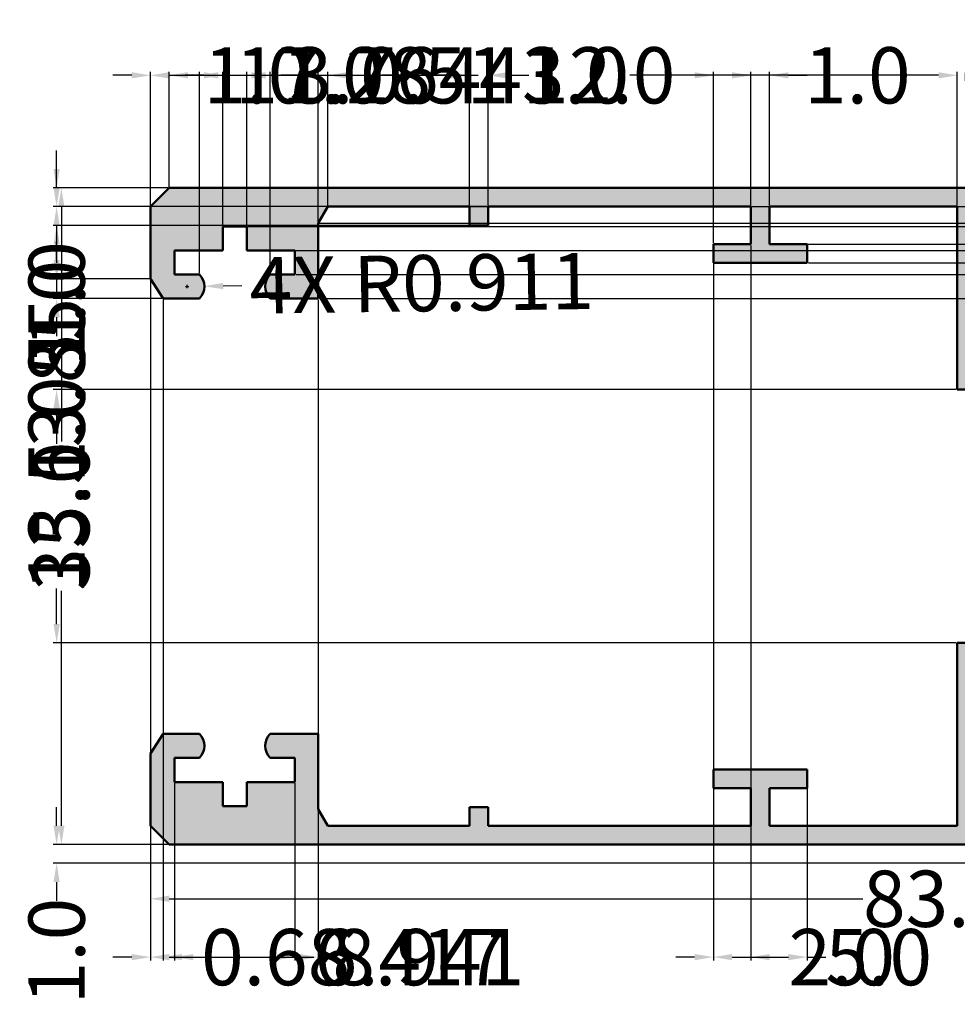
# Model space of a CAD drawing. Units: millimetres. Extents: x 9 to 262, y -226 to 104.
# Tile 3 of 4: x 119 to 169, y 13 to 66. Entities that reach past the tile are written whole.
import ezdxf

# ---------------------------------------------------------------- set-up
doc = ezdxf.new("R2010")
doc.units = ezdxf.units.MM
doc.header["$MEASUREMENT"] = 0
for name, color, linetype, lineweight in [('M-DIMS', 2, 'Continuous', 25), ('M-HATC', 9, 'Continuous', 18), ('M-OUTL', 7, 'Continuous', 50)]:
    doc.layers.add(name, color=color, linetype=linetype, lineweight=lineweight)
doc.styles.get("Standard").update_dxf_attribs({"font": 'arial.ttf'})
doc.dimstyles.get("Standard").update_dxf_attribs({"dimtxt": 3, "dimasz": 1, "dimexe": 0.18, "dimexo": 0.0625, "dimgap": 0.09, "dimtad": 0, "dimdec": 1, "dimzin": 0, "dimdsep": 46, "dimtxsty": 'Standard', "dimcen": 0.09, "dimadec": 0, "dimazin": 0, "dimtfac": 1, "dimtdec": 1, "dimtofl": 0, "dimtmove": 0, "dimatfit": 3, "dimfxl": 1, "dimtolj": 1, "dimtzin": 0, "dimarcsym": 0})

# ---------------------------------------------------------------- blocks, each defined once
blk = doc.blocks.new('*D3')
at = {"layer": 'Defpoints', "color": 0, "transparency": 16777216}
for p in [(126.103, 21.114), (210.003, 21.345), (126.103, 18.955)]:
    blk.add_point(p, dxfattribs=at)
at = {"layer": 'M-DIMS', "color": 0, "lineweight": -2, "transparency": 16777216}
for p, q in [((126.103, 21.051), (126.103, 18.775)), ((210.003, 21.282), (210.003, 18.775)), ((127.103, 18.955), (164.062, 18.955)), ((209.003, 18.955), (172.045, 18.955))]:
    blk.add_line(p, q, dxfattribs=at)
at = {"layer": 'M-DIMS', "color": 0, "transparency": 16777216}
for points in [[(127.103, 19.122), (127.103, 18.788), (126.103, 18.955)], [(209.003, 19.122), (209.003, 18.788), (210.003, 18.955)]]:
    blk.add_solid(points, dxfattribs=at)
at = {"layer": 'M-DIMS', "color": 0, "transparency": 16777216, "insert": (168.053, 18.955), "char_height": 3, "attachment_point": 5}
blk.add_mtext('\\A1;83.9', dxfattribs=at)
blk = doc.blocks.new('*D4')
at = {"layer": 'Defpoints', "color": 0, "transparency": 16777216}
for p in [(127.103, 56.845), (121.354, 21.845), (127.103, 21.845)]:
    blk.add_point(p, dxfattribs=at)
at = {"layer": 'M-DIMS', "color": 0, "lineweight": -2, "transparency": 16777216}
for p, q in [((127.041, 56.845), (121.174, 56.845)), ((121.354, 55.845), (121.354, 43.325)), ((121.354, 22.845), (121.354, 35.365)), ((127.041, 21.845), (121.174, 21.845))]:
    blk.add_line(p, q, dxfattribs=at)
at = {"layer": 'M-DIMS', "color": 0, "transparency": 16777216}
for points in [[(121.188, 55.845), (121.521, 55.845), (121.354, 56.845)], [(121.188, 22.845), (121.521, 22.845), (121.354, 21.845)]]:
    blk.add_solid(points, dxfattribs=at)
at = {"layer": 'M-DIMS', "color": 0, "transparency": 16777216, "insert": (121.354, 39.345), "char_height": 3, "attachment_point": 5, "rotation": 90}
blk.add_mtext('\\A1;35.0', dxfattribs=at)
blk = doc.blocks.new('PROFILE-SASH')
for p, q in [((66.477, 36), (68.209, 37)), ((68.209, 37), (83.4, 37)), ((1, 36), (0, 35)), ((1, 36), (66.477, 36)), ((68, 35.724), (68.477, 36)), ((68, 35.724), (68, 1.275)), ((68.477, 36), (75.189, 36)), ((75.189, 36), (75.189, 33.5)), ((76.189, 36), (76.189, 33.5)), ((76.189, 36), (81.9, 36)), ((81.9, 36), (81.9, 32)), ((82.9, 36), (82.9, 32)), ((82.9, 36), (83.4, 36)), ((0, 35), (0, 31.15)), ((8.941, 34.12), (9.449, 35)), ((9.449, 35), (17, 35)), ((17, 35), (17, 34)), ((18, 35), (18, 34)), ((18, 35), (32, 35)), ((32, 35), (32, 33)), ((33, 35), (33, 33)), ((33, 35), (33, 33)), ((33, 35), (43, 35)), ((43, 35), (43, 25.25)), ((44, 35), (44, 28.25)), ((44, 35), (54, 35)), ((54, 35), (54, 34.5)), ((55, 35), (55, 34.5)), ((55, 35), (67, 35)), ((55, 35), (66.477, 35)), ((67, 35), (67, 2)), ((8.941, 30.101), (8.941, 34.12)), ((3.851, 32.668), (3.851, 33.951)), ((3.851, 33.951), (5.134, 33.951)), ((5.134, 32.668), (5.134, 33.951)), ((17, 34), (18, 34)), ((1.284, 31.384), (1.284, 32.668)), ((1.284, 31.384), (1.284, 32.668)), ((1.284, 32.668), (3.851, 32.668)), ((7.701, 32.668), (5.134, 32.668)), ((7.701, 31.384), (7.701, 32.668)), ((30, 32), (30, 33)), ((30, 33), (32, 33)), ((33, 33), (35, 33)), ((35, 33), (35, 32)), ((32, 32), (30, 32)), ((35, 32), (32, 32)), ((0, 31.15), (0.685, 30.101)), ((2.61, 31.384), (1.284, 31.384)), ((6.374, 31.384), (7.701, 31.384)), ((0.685, 30.101), (2.61, 30.101)), ((6.374, 30.101), (8.941, 30.101)), ((44, 28.25), (49, 28.25)), ((49, 28.25), (49, 8.75)), ((44, 27.25), (48, 27.25)), ((44, 27.25), (44, 25.25)), ((48, 27.25), (48, 9.75)), ((43, 25.25), (44, 25.25)), ((43, 11.75), (44, 11.75)), ((43, 11.75), (43, 2)), ((44, 11.75), (44, 9.75)), ((48, 9.75), (44, 9.75)), ((49, 8.75), (44, 8.75)), ((44, 8.75), (44, 2)), ((0, 5.85), (0.685, 6.899)), ((0.685, 6.899), (2.61, 6.899)), ((6.374, 6.899), (8.941, 6.899)), ((8.941, 6.899), (8.941, 2.879)), ((0, 5.85), (0, 2)), ((1.284, 5.615), (1.284, 4.332)), ((2.61, 5.615), (1.284, 5.615)), ((1.284, 5.615), (1.284, 4.332)), ((6.374, 5.615), (7.701, 5.615)), ((7.701, 5.615), (7.701, 4.332)), ((32, 5), (30, 5)), ((30, 5), (30, 4)), ((35, 5), (32, 5)), ((35, 4), (35, 5)), ((81.9, 5), (81.9, 1)), ((82.9, 5), (82.9, 1)), ((1.284, 4.332), (3.851, 4.332)), ((3.851, 4.332), (3.851, 3.049)), ((7.701, 4.332), (5.134, 4.332)), ((5.134, 4.332), (5.134, 3.049)), ((30, 4), (32, 4)), ((32, 4), (32, 2)), ((33, 2), (33, 4)), ((33, 4), (35, 4)), ((33, 4), (33, 2)), ((75.189, 3.5), (75.189, 1)), ((76.189, 3.5), (76.189, 1)), ((3.851, 3.049), (5.134, 3.049)), ((8.941, 2.879), (9.449, 2)), ((17, 3), (18, 3)), ((17, 3), (17, 2)), ((18, 3), (18, 2)), ((54, 2.5), (54, 2)), ((55, 2.5), (55, 2)), ((0, 2), (1, 1)), ((9.449, 2), (17, 2)), ((18, 2), (32, 2)), ((33, 2), (43, 2)), ((44, 2), (54, 2)), ((44, 2), (54, 2)), ((55, 2), (67, 2)), ((55, 2), (66.477, 2)), ((68, 1.275), (68.477, 1)), ((1, 1), (66.477, 1)), ((66.477, 1), (68.209, 0)), ((68.477, 1), (75.189, 1)), ((76.189, 1), (81.9, 1)), ((76.189, 1), (81.9, 1)), ((82.9, 1), (83.4, 1)), ((82.9, 1), (83.4, 1)), ((68.209, 0), (83.4, 0))]:
    blk.add_line(p, q)
for centre, radius, start, end in [((83.4, 36.5), 0.5, 270, 90), ((54.5, 34.5), 0.5, 180, 0), ((75.689, 33.5), 0.5, 180, 0), ((82.4, 32), 0.5, 180, 0), ((1.964, 30.743), 0.911, 315.2177, 44.7823), ((7.021, 30.743), 0.911, 135.2177, 224.7823), ((1.964, 6.257), 0.911, 315.2177, 44.7823), ((7.021, 6.257), 0.911, 135.2177, 224.7823), ((82.4, 5), 0.5, 0, 180), ((75.689, 3.5), 0.5, 0, 180), ((54.5, 2.5), 0.5, 0, 180), ((83.4, 0.5), 0.5, 270, 90)]:
    blk.add_arc(centre, radius, start, end)
blk = doc.blocks.new('*D20')
at = {"layer": 'Defpoints', "color": 0, "transparency": 16777216}
for p in [(169.103, 62.845), (126.103, 55.845), (169.103, 55.845)]:
    blk.add_point(p, dxfattribs=at)
at = {"layer": 'M-DIMS', "color": 0, "lineweight": -2, "transparency": 16777216}
for p, q in [((126.103, 55.907), (126.103, 63.025)), ((169.103, 55.907), (169.103, 63.025)), ((127.103, 62.845), (143.562, 62.845)), ((168.103, 62.845), (151.645, 62.845))]:
    blk.add_line(p, q, dxfattribs=at)
at = {"layer": 'M-DIMS', "color": 0, "transparency": 16777216}
for points in [[(127.103, 63.012), (127.103, 62.678), (126.103, 62.845)], [(168.103, 63.012), (168.103, 62.678), (169.103, 62.845)]]:
    blk.add_solid(points, dxfattribs=at)
at = {"layer": 'M-DIMS', "color": 0, "transparency": 16777216, "insert": (147.603, 62.845), "char_height": 3, "attachment_point": 5}
blk.add_mtext('\\A1;43.0', dxfattribs=at)
blk = doc.blocks.new('*D21')
at = {"layer": 'Defpoints', "color": 0, "transparency": 16777216}
for p in [(175.103, 62.845), (169.103, 55.845), (175.103, 49.095)]:
    blk.add_point(p, dxfattribs=at)
at = {"layer": 'M-DIMS', "color": 0, "lineweight": -2, "transparency": 16777216}
for p, q in [((169.103, 55.907), (169.103, 63.025)), ((175.103, 49.157), (175.103, 63.025)), ((168.103, 62.845), (167.103, 62.845)), ((176.103, 62.845), (177.103, 62.845))]:
    blk.add_line(p, q, dxfattribs=at)
at = {"layer": 'M-DIMS', "color": 0, "transparency": 16777216}
for points in [[(168.103, 63.012), (168.103, 62.678), (169.103, 62.845)], [(176.103, 63.012), (176.103, 62.678), (175.103, 62.845)]]:
    blk.add_solid(points, dxfattribs=at)
at = {"layer": 'M-DIMS', "color": 0, "transparency": 16777216, "insert": (172.103, 62.845), "char_height": 3, "attachment_point": 5}
blk.add_mtext('\\A1;6.0', dxfattribs=at)
blk = doc.blocks.new('*D28')
at = {"layer": 'Defpoints', "color": 0, "transparency": 16777216}
for p in [(127.103, 56.845), (121.103, 55.845), (135.552, 55.845)]:
    blk.add_point(p, dxfattribs=at)
at = {"layer": 'M-DIMS', "color": 0, "lineweight": -2, "transparency": 16777216}
for p, q in [((121.103, 57.845), (121.103, 58.845)), ((127.041, 56.845), (120.923, 56.845)), ((135.49, 55.845), (120.923, 55.845)), ((121.103, 54.845), (121.103, 53.845))]:
    blk.add_line(p, q, dxfattribs=at)
at = {"layer": 'M-DIMS', "color": 0, "transparency": 16777216}
for points in [[(120.937, 57.845), (121.27, 57.845), (121.103, 56.845)], [(120.937, 54.845), (121.27, 54.845), (121.103, 55.845)]]:
    blk.add_solid(points, dxfattribs=at)
at = {"layer": 'M-DIMS', "color": 0, "transparency": 16777216, "insert": (121.103, 51.17), "char_height": 3, "attachment_point": 5, "rotation": 90}
blk.add_mtext('\\A1;1.0', dxfattribs=at)
blk = doc.blocks.new('*D29')
at = {"layer": 'Defpoints', "color": 0, "transparency": 16777216}
for p in [(127.387, 25.177), (133.804, 25.177), (133.804, 15.845)]:
    blk.add_point(p, dxfattribs=at)
at = {"layer": 'M-DIMS', "color": 0, "lineweight": -2, "transparency": 16777216}
for p, q in [((127.387, 25.115), (127.387, 15.665)), ((133.804, 25.115), (133.804, 15.665)), ((128.387, 15.845), (132.804, 15.845)), ((133.804, 15.845), (134.804, 15.845))]:
    blk.add_line(p, q, dxfattribs=at)
at = {"layer": 'M-DIMS', "color": 0, "transparency": 16777216}
for points in [[(128.387, 16.012), (128.387, 15.678), (127.387, 15.845)], [(132.804, 16.012), (132.804, 15.678), (133.804, 15.845)]]:
    blk.add_solid(points, dxfattribs=at)
at = {"layer": 'M-DIMS', "color": 0, "transparency": 16777216, "insert": (139.964, 15.845), "char_height": 3, "attachment_point": 5}
blk.add_mtext('\\A1;6.417', dxfattribs=at)
blk = doc.blocks.new('*D30')
at = {"layer": 'Defpoints', "color": 0, "transparency": 16777216}
for p in [(156.103, 25.845), (161.103, 25.845), (161.103, 15.845)]:
    blk.add_point(p, dxfattribs=at)
at = {"layer": 'M-DIMS', "color": 0, "lineweight": -2, "transparency": 16777216}
for p, q in [((156.103, 25.782), (156.103, 15.665)), ((161.103, 25.782), (161.103, 15.665)), ((157.103, 15.845), (160.103, 15.845)), ((161.103, 15.845), (162.103, 15.845))]:
    blk.add_line(p, q, dxfattribs=at)
at = {"layer": 'M-DIMS', "color": 0, "transparency": 16777216}
for points in [[(157.103, 16.012), (157.103, 15.678), (156.103, 15.845)], [(160.103, 16.012), (160.103, 15.678), (161.103, 15.845)]]:
    blk.add_solid(points, dxfattribs=at)
at = {"layer": 'M-DIMS', "color": 0, "transparency": 16777216, "insert": (164.919, 15.845), "char_height": 3, "attachment_point": 5}
blk.add_mtext('\\A1;5.0', dxfattribs=at)
blk = doc.blocks.new('*D46')
at = {"layer": 'Defpoints', "color": 0, "transparency": 16777216}
for p in [(127.103, 62.845), (127.103, 56.845), (126.103, 55.845)]:
    blk.add_point(p, dxfattribs=at)
at = {"layer": 'M-DIMS', "color": 0, "lineweight": -2, "transparency": 16777216}
for p, q in [((126.103, 55.907), (126.103, 63.025)), ((127.103, 56.907), (127.103, 63.025)), ((125.103, 62.845), (124.103, 62.845)), ((128.103, 62.845), (129.103, 62.845))]:
    blk.add_line(p, q, dxfattribs=at)
at = {"layer": 'M-DIMS', "color": 0, "transparency": 16777216}
for points in [[(125.103, 63.012), (125.103, 62.678), (126.103, 62.845)], [(128.103, 63.012), (128.103, 62.678), (127.103, 62.845)]]:
    blk.add_solid(points, dxfattribs=at)
at = {"layer": 'M-DIMS', "color": 0, "transparency": 16777216, "insert": (131.778, 62.845), "char_height": 3, "attachment_point": 5}
blk.add_mtext('\\A1;1.0', dxfattribs=at)
blk = doc.blocks.new('*D47')
at = {"layer": 'Defpoints', "color": 0, "transparency": 16777216}
for p in [(135.552, 62.845), (135.552, 55.845), (135.044, 54.965)]:
    blk.add_point(p, dxfattribs=at)
at = {"layer": 'M-DIMS', "color": 0, "lineweight": -2, "transparency": 16777216}
for p, q in [((135.044, 55.028), (135.044, 63.025)), ((135.552, 55.907), (135.552, 63.025)), ((134.044, 62.845), (133.044, 62.845)), ((136.552, 62.845), (137.552, 62.845))]:
    blk.add_line(p, q, dxfattribs=at)
at = {"layer": 'M-DIMS', "color": 0, "transparency": 16777216}
for points in [[(134.044, 63.012), (134.044, 62.678), (135.044, 62.845)], [(136.552, 63.012), (136.552, 62.678), (135.552, 62.845)]]:
    blk.add_solid(points, dxfattribs=at)
at = {"layer": 'M-DIMS', "color": 0, "transparency": 16777216, "insert": (141.249, 62.845), "char_height": 3, "attachment_point": 5}
blk.add_mtext('\\A1;0.51', dxfattribs=at)
blk = doc.blocks.new('*D48')
at = {"layer": 'Defpoints', "color": 0, "transparency": 16777216}
for p in [(135.552, 55.845), (215.003, 55.845), (135.044, 54.965)]:
    blk.add_point(p, dxfattribs=at)
at = {"layer": 'M-DIMS', "color": 0, "lineweight": -2, "transparency": 16777216}
for p, q in [((215.003, 56.845), (215.003, 57.845)), ((135.615, 55.845), (215.183, 55.845)), ((135.107, 54.965), (215.183, 54.965)), ((215.003, 53.965), (215.003, 52.965))]:
    blk.add_line(p, q, dxfattribs=at)
at = {"layer": 'M-DIMS', "color": 0, "transparency": 16777216}
for points in [[(214.837, 56.845), (215.17, 56.845), (215.003, 55.845)], [(214.837, 53.965), (215.17, 53.965), (215.003, 54.965)]]:
    blk.add_solid(points, dxfattribs=at)
at = {"layer": 'M-DIMS', "color": 0, "transparency": 16777216, "insert": (215.003, 61.834), "char_height": 3, "attachment_point": 5, "rotation": 90}
blk.add_mtext('\\A1;0.88', dxfattribs=at)
blk = doc.blocks.new('*D49')
at = {"layer": 'Defpoints', "color": 0, "transparency": 16777216}
for p in [(126.103, 51.995), (126.788, 50.946), (126.788, 15.845)]:
    blk.add_point(p, dxfattribs=at)
at = {"layer": 'M-DIMS', "color": 0, "lineweight": -2, "transparency": 16777216}
for p, q in [((126.103, 51.932), (126.103, 15.665)), ((126.788, 50.883), (126.788, 15.665)), ((125.103, 15.845), (124.103, 15.845)), ((127.788, 15.845), (128.788, 15.845))]:
    blk.add_line(p, q, dxfattribs=at)
at = {"layer": 'M-DIMS', "color": 0, "transparency": 16777216}
for points in [[(125.103, 16.012), (125.103, 15.678), (126.103, 15.845)], [(127.788, 16.012), (127.788, 15.678), (126.788, 15.845)]]:
    blk.add_solid(points, dxfattribs=at)
at = {"layer": 'M-DIMS', "color": 0, "transparency": 16777216, "insert": (132.778, 15.845), "char_height": 3, "attachment_point": 5}
blk.add_mtext('\\A1;0.68', dxfattribs=at)
blk = doc.blocks.new('*D50')
at = {"layer": 'Defpoints', "color": 0, "transparency": 16777216}
for p in [(126.103, 55.845), (121.103, 51.995), (126.103, 51.995)]:
    blk.add_point(p, dxfattribs=at)
at = {"layer": 'M-DIMS', "color": 0, "lineweight": -2, "transparency": 16777216}
for p, q in [((126.041, 55.845), (120.923, 55.845)), ((121.103, 54.845), (121.103, 52.995)), ((126.041, 51.995), (120.923, 51.995)), ((121.103, 51.995), (121.103, 50.995))]:
    blk.add_line(p, q, dxfattribs=at)
at = {"layer": 'M-DIMS', "color": 0, "transparency": 16777216}
for points in [[(120.937, 54.845), (121.27, 54.845), (121.103, 55.845)], [(120.937, 52.995), (121.27, 52.995), (121.103, 51.995)]]:
    blk.add_solid(points, dxfattribs=at)
at = {"layer": 'M-DIMS', "color": 0, "transparency": 16777216, "insert": (121.103, 46.998), "char_height": 3, "attachment_point": 5, "rotation": 90}
blk.add_mtext('\\A1;3.85', dxfattribs=at)
blk = doc.blocks.new('*D51')
at = {"layer": 'Defpoints', "color": 0, "transparency": 16777216}
for p in [(126.103, 51.995), (121.103, 50.946), (126.788, 50.946)]:
    blk.add_point(p, dxfattribs=at)
at = {"layer": 'M-DIMS', "color": 0, "lineweight": -2, "transparency": 16777216}
for p, q in [((121.103, 52.995), (121.103, 53.995)), ((126.041, 51.995), (120.923, 51.995)), ((126.726, 50.946), (120.923, 50.946)), ((121.103, 49.946), (121.103, 48.946))]:
    blk.add_line(p, q, dxfattribs=at)
at = {"layer": 'M-DIMS', "color": 0, "transparency": 16777216}
for points in [[(120.937, 52.995), (121.27, 52.995), (121.103, 51.995)], [(120.937, 49.946), (121.27, 49.946), (121.103, 50.946)]]:
    blk.add_solid(points, dxfattribs=at)
at = {"layer": 'M-DIMS', "color": 0, "transparency": 16777216, "insert": (121.103, 45.089), "char_height": 3, "attachment_point": 5, "rotation": 90}
blk.add_mtext('\\A1;1.05', dxfattribs=at)
blk = doc.blocks.new('*D52')
at = {"layer": 'Defpoints', "color": 0, "transparency": 16777216}
for p in [(133.804, 53.513), (215.003, 53.513), (135.044, 50.946)]:
    blk.add_point(p, dxfattribs=at)
at = {"layer": 'M-DIMS', "color": 0, "lineweight": -2, "transparency": 16777216}
for p, q in [((215.003, 53.513), (215.003, 54.513)), ((133.867, 53.513), (215.183, 53.513)), ((215.003, 51.946), (215.003, 52.513)), ((135.107, 50.946), (215.183, 50.946))]:
    blk.add_line(p, q, dxfattribs=at)
at = {"layer": 'M-DIMS', "color": 0, "transparency": 16777216}
for points in [[(214.837, 52.513), (215.17, 52.513), (215.003, 53.513)], [(214.837, 51.946), (215.17, 51.946), (215.003, 50.946)]]:
    blk.add_solid(points, dxfattribs=at)
at = {"layer": 'M-DIMS', "color": 0, "transparency": 16777216, "insert": (215.003, 59.69), "char_height": 3, "attachment_point": 5, "rotation": 90}
blk.add_mtext('\\A1;2.567', dxfattribs=at)
blk = doc.blocks.new('*D53')
at = {"layer": 'Defpoints', "color": 0, "transparency": 16777216}
for p in [(133.804, 53.513), (215.003, 53.513), (133.804, 52.229)]:
    blk.add_point(p, dxfattribs=at)
at = {"layer": 'M-DIMS', "color": 0, "lineweight": -2, "transparency": 16777216}
for p, q in [((215.003, 54.513), (215.003, 55.513)), ((133.867, 53.513), (215.183, 53.513)), ((133.867, 52.229), (215.183, 52.229)), ((215.003, 51.229), (215.003, 50.229))]:
    blk.add_line(p, q, dxfattribs=at)
at = {"layer": 'M-DIMS', "color": 0, "transparency": 16777216}
for points in [[(214.837, 54.513), (215.17, 54.513), (215.003, 53.513)], [(214.837, 51.229), (215.17, 51.229), (215.003, 52.229)]]:
    blk.add_solid(points, dxfattribs=at)
at = {"layer": 'M-DIMS', "color": 0, "transparency": 16777216, "insert": (215.003, 59.361), "char_height": 3, "attachment_point": 5, "rotation": 90}
blk.add_mtext('\\A1;1.28', dxfattribs=at)
blk = doc.blocks.new('*D54')
at = {"layer": 'Defpoints', "color": 0, "transparency": 16777216}
for p in [(131.237, 54.796), (215.003, 54.796), (131.237, 53.513)]:
    blk.add_point(p, dxfattribs=at)
at = {"layer": 'M-DIMS', "color": 0, "lineweight": -2, "transparency": 16777216}
for p, q in [((215.003, 55.796), (215.003, 56.796)), ((131.3, 54.796), (215.183, 54.796)), ((131.3, 53.513), (215.183, 53.513)), ((215.003, 52.513), (215.003, 51.513))]:
    blk.add_line(p, q, dxfattribs=at)
at = {"layer": 'M-DIMS', "color": 0, "transparency": 16777216}
for points in [[(214.837, 55.796), (215.17, 55.796), (215.003, 54.796)], [(214.837, 52.513), (215.17, 52.513), (215.003, 53.513)]]:
    blk.add_solid(points, dxfattribs=at)
at = {"layer": 'M-DIMS', "color": 0, "transparency": 16777216, "insert": (215.003, 60.644), "char_height": 3, "attachment_point": 5, "rotation": 90}
blk.add_mtext('\\A1;1.28', dxfattribs=at)
blk = doc.blocks.new('*D55')
at = {"layer": 'Defpoints', "color": 0, "transparency": 16777216}
for p in [(132.477, 62.845), (128.713, 52.229), (132.477, 52.229)]:
    blk.add_point(p, dxfattribs=at)
at = {"layer": 'M-DIMS', "color": 0, "lineweight": -2, "transparency": 16777216}
for p, q in [((128.713, 52.292), (128.713, 63.025)), ((132.477, 52.292), (132.477, 63.025)), ((129.713, 62.845), (131.477, 62.845)), ((132.477, 62.845), (133.477, 62.845))]:
    blk.add_line(p, q, dxfattribs=at)
at = {"layer": 'M-DIMS', "color": 0, "transparency": 16777216}
for points in [[(129.713, 63.012), (129.713, 62.678), (128.713, 62.845)], [(131.477, 63.012), (131.477, 62.678), (132.477, 62.845)]]:
    blk.add_solid(points, dxfattribs=at)
at = {"layer": 'M-DIMS', "color": 0, "transparency": 16777216, "insert": (138.622, 62.845), "char_height": 3, "attachment_point": 5}
blk.add_mtext('\\A1;3.764', dxfattribs=at)
blk = doc.blocks.new('*D56')
at = {"layer": 'Defpoints', "color": 0, "transparency": 16777216}
for p in [(131.237, 62.845), (129.954, 54.796), (131.237, 54.796)]:
    blk.add_point(p, dxfattribs=at)
at = {"layer": 'M-DIMS', "color": 0, "lineweight": -2, "transparency": 16777216}
for p, q in [((129.954, 54.859), (129.954, 63.025)), ((131.237, 54.859), (131.237, 63.025)), ((128.954, 62.845), (127.954, 62.845)), ((132.237, 62.845), (133.237, 62.845))]:
    blk.add_line(p, q, dxfattribs=at)
at = {"layer": 'M-DIMS', "color": 0, "transparency": 16777216}
for points in [[(128.954, 63.012), (128.954, 62.678), (129.954, 62.845)], [(132.237, 63.012), (132.237, 62.678), (131.237, 62.845)]]:
    blk.add_solid(points, dxfattribs=at)
at = {"layer": 'M-DIMS', "color": 0, "transparency": 16777216, "insert": (137.085, 62.845), "char_height": 3, "attachment_point": 5}
blk.add_mtext('\\A1;1.28', dxfattribs=at)
blk = doc.blocks.new('*D57')
at = {"layer": 'Defpoints', "color": 0, "transparency": 16777216}
for p in [(126.103, 51.995), (135.044, 50.946), (135.044, 15.845)]:
    blk.add_point(p, dxfattribs=at)
at = {"layer": 'M-DIMS', "color": 0, "lineweight": -2, "transparency": 16777216}
for p, q in [((126.103, 51.932), (126.103, 15.665)), ((135.044, 50.883), (135.044, 15.665)), ((127.103, 15.845), (134.044, 15.845)), ((135.044, 15.845), (136.044, 15.845))]:
    blk.add_line(p, q, dxfattribs=at)
at = {"layer": 'M-DIMS', "color": 0, "transparency": 16777216}
for points in [[(127.103, 16.012), (127.103, 15.678), (126.103, 15.845)], [(134.044, 16.012), (134.044, 15.678), (135.044, 15.845)]]:
    blk.add_solid(points, dxfattribs=at)
at = {"layer": 'M-DIMS', "color": 0, "transparency": 16777216, "insert": (140.909, 15.845), "char_height": 3, "attachment_point": 5}
blk.add_mtext('\\A1;8.941', dxfattribs=at)
blk = doc.blocks.new('*D58')
at = {"layer": 'Defpoints', "color": 0, "transparency": 16777216}
for p in [(143.103, 62.845), (126.103, 55.845), (143.103, 55.845)]:
    blk.add_point(p, dxfattribs=at)
at = {"layer": 'M-DIMS', "color": 0, "lineweight": -2, "transparency": 16777216}
for p, q in [((126.103, 55.907), (126.103, 63.025)), ((143.103, 55.907), (143.103, 63.025)), ((127.103, 62.845), (130.763, 62.845)), ((142.103, 62.845), (138.443, 62.845))]:
    blk.add_line(p, q, dxfattribs=at)
at = {"layer": 'M-DIMS', "color": 0, "transparency": 16777216}
for points in [[(127.103, 63.012), (127.103, 62.678), (126.103, 62.845)], [(142.103, 63.012), (142.103, 62.678), (143.103, 62.845)]]:
    blk.add_solid(points, dxfattribs=at)
at = {"layer": 'M-DIMS', "color": 0, "transparency": 16777216, "insert": (134.603, 62.845), "char_height": 3, "attachment_point": 5}
blk.add_mtext('\\A1;17.0', dxfattribs=at)
blk = doc.blocks.new('*D59')
at = {"layer": 'Defpoints', "color": 0, "transparency": 16777216}
for p in [(144.103, 62.845), (143.103, 55.845), (144.103, 55.845)]:
    blk.add_point(p, dxfattribs=at)
at = {"layer": 'M-DIMS', "color": 0, "lineweight": -2, "transparency": 16777216}
for p, q in [((143.103, 55.907), (143.103, 63.025)), ((144.103, 55.907), (144.103, 63.025)), ((142.103, 62.845), (141.103, 62.845)), ((145.103, 62.845), (146.103, 62.845))]:
    blk.add_line(p, q, dxfattribs=at)
at = {"layer": 'M-DIMS', "color": 0, "transparency": 16777216}
for points in [[(142.103, 63.012), (142.103, 62.678), (143.103, 62.845)], [(145.103, 63.012), (145.103, 62.678), (144.103, 62.845)]]:
    blk.add_solid(points, dxfattribs=at)
at = {"layer": 'M-DIMS', "color": 0, "transparency": 16777216, "insert": (148.778, 62.845), "char_height": 3, "attachment_point": 5}
blk.add_mtext('\\A1;1.0', dxfattribs=at)
blk = doc.blocks.new('*D60')
at = {"layer": 'Defpoints', "color": 0, "transparency": 16777216}
for p in [(156.103, 62.845), (144.103, 55.845), (156.103, 53.845)]:
    blk.add_point(p, dxfattribs=at)
at = {"layer": 'M-DIMS', "color": 0, "lineweight": -2, "transparency": 16777216}
for p, q in [((144.103, 55.907), (144.103, 63.025)), ((156.103, 53.907), (156.103, 63.025)), ((145.103, 62.845), (146.263, 62.845)), ((155.103, 62.845), (153.943, 62.845))]:
    blk.add_line(p, q, dxfattribs=at)
at = {"layer": 'M-DIMS', "color": 0, "transparency": 16777216}
for points in [[(145.103, 63.012), (145.103, 62.678), (144.103, 62.845)], [(155.103, 63.012), (155.103, 62.678), (156.103, 62.845)]]:
    blk.add_solid(points, dxfattribs=at)
at = {"layer": 'M-DIMS', "color": 0, "transparency": 16777216, "insert": (150.103, 62.845), "char_height": 3, "attachment_point": 5}
blk.add_mtext('\\A1;12.0', dxfattribs=at)
blk = doc.blocks.new('*D61')
at = {"layer": 'Defpoints', "color": 0, "transparency": 16777216}
for p in [(144.103, 55.845), (121.103, 54.845), (144.103, 54.845)]:
    blk.add_point(p, dxfattribs=at)
at = {"layer": 'M-DIMS', "color": 0, "lineweight": -2, "transparency": 16777216}
for p, q in [((121.103, 56.845), (121.103, 57.845)), ((144.041, 55.845), (120.923, 55.845)), ((144.041, 54.845), (120.923, 54.845)), ((121.103, 53.845), (121.103, 52.845))]:
    blk.add_line(p, q, dxfattribs=at)
at = {"layer": 'M-DIMS', "color": 0, "transparency": 16777216}
for points in [[(120.937, 56.845), (121.27, 56.845), (121.103, 55.845)], [(120.937, 53.845), (121.27, 53.845), (121.103, 54.845)]]:
    blk.add_solid(points, dxfattribs=at)
at = {"layer": 'M-DIMS', "color": 0, "transparency": 16777216, "insert": (121.103, 50.17), "char_height": 3, "attachment_point": 5, "rotation": 90}
blk.add_mtext('\\A1;1.0', dxfattribs=at)
blk = doc.blocks.new('*D62')
at = {"layer": 'Defpoints', "color": 0, "transparency": 16777216}
for p in [(159.103, 62.845), (158.103, 55.845), (159.103, 55.845)]:
    blk.add_point(p, dxfattribs=at)
at = {"layer": 'M-DIMS', "color": 0, "lineweight": -2, "transparency": 16777216}
for p, q in [((158.103, 55.907), (158.103, 63.025)), ((159.103, 55.907), (159.103, 63.025)), ((157.103, 62.845), (156.103, 62.845)), ((160.103, 62.845), (161.103, 62.845))]:
    blk.add_line(p, q, dxfattribs=at)
at = {"layer": 'M-DIMS', "color": 0, "transparency": 16777216}
for points in [[(157.103, 63.012), (157.103, 62.678), (158.103, 62.845)], [(160.103, 63.012), (160.103, 62.678), (159.103, 62.845)]]:
    blk.add_solid(points, dxfattribs=at)
at = {"layer": 'M-DIMS', "color": 0, "transparency": 16777216, "insert": (163.778, 62.845), "char_height": 3, "attachment_point": 5}
blk.add_mtext('\\A1;1.0', dxfattribs=at)
blk = doc.blocks.new('*D63')
at = {"layer": 'Defpoints', "color": 0, "transparency": 16777216}
for p in [(156.103, 53.845), (158.103, 53.845), (158.103, 15.845)]:
    blk.add_point(p, dxfattribs=at)
at = {"layer": 'M-DIMS', "color": 0, "lineweight": -2, "transparency": 16777216}
for p, q in [((156.103, 53.782), (156.103, 15.665)), ((158.103, 53.782), (158.103, 15.665)), ((155.103, 15.845), (154.103, 15.845)), ((159.103, 15.845), (160.103, 15.845))]:
    blk.add_line(p, q, dxfattribs=at)
at = {"layer": 'M-DIMS', "color": 0, "transparency": 16777216}
for points in [[(155.103, 16.012), (155.103, 15.678), (156.103, 15.845)], [(159.103, 16.012), (159.103, 15.678), (158.103, 15.845)]]:
    blk.add_solid(points, dxfattribs=at)
at = {"layer": 'M-DIMS', "color": 0, "transparency": 16777216, "insert": (162.945, 15.845), "char_height": 3, "attachment_point": 5}
blk.add_mtext('\\A1;2.0', dxfattribs=at)
blk = doc.blocks.new('*D64')
at = {"layer": 'Defpoints', "color": 0, "transparency": 16777216}
for p in [(159.103, 55.845), (159.103, 53.845), (215.003, 53.845)]:
    blk.add_point(p, dxfattribs=at)
at = {"layer": 'M-DIMS', "color": 0, "lineweight": -2, "transparency": 16777216}
for p, q in [((215.003, 56.845), (215.003, 57.845)), ((159.166, 55.845), (215.183, 55.845)), ((159.166, 53.845), (215.183, 53.845)), ((215.003, 52.845), (215.003, 51.845))]:
    blk.add_line(p, q, dxfattribs=at)
at = {"layer": 'M-DIMS', "color": 0, "transparency": 16777216}
for points in [[(214.837, 56.845), (215.17, 56.845), (215.003, 55.845)], [(214.837, 52.845), (215.17, 52.845), (215.003, 53.845)]]:
    blk.add_solid(points, dxfattribs=at)
at = {"layer": 'M-DIMS', "color": 0, "transparency": 16777216, "insert": (215.003, 49.004), "char_height": 3, "attachment_point": 5, "rotation": 90}
blk.add_mtext('\\A1;2.0', dxfattribs=at)
blk = doc.blocks.new('*D65')
at = {"layer": 'Defpoints', "color": 0, "transparency": 16777216}
for p in [(161.103, 53.845), (161.103, 52.845), (215.003, 52.845)]:
    blk.add_point(p, dxfattribs=at)
at = {"layer": 'M-DIMS', "color": 0, "lineweight": -2, "transparency": 16777216}
for p, q in [((215.003, 54.845), (215.003, 55.845)), ((161.166, 53.845), (215.183, 53.845)), ((161.166, 52.845), (215.183, 52.845)), ((215.003, 51.845), (215.003, 50.845))]:
    blk.add_line(p, q, dxfattribs=at)
at = {"layer": 'M-DIMS', "color": 0, "transparency": 16777216}
for points in [[(214.837, 54.845), (215.17, 54.845), (215.003, 53.845)], [(214.837, 51.845), (215.17, 51.845), (215.003, 52.845)]]:
    blk.add_solid(points, dxfattribs=at)
at = {"layer": 'M-DIMS', "color": 0, "transparency": 16777216, "insert": (215.003, 48.17), "char_height": 3, "attachment_point": 5, "rotation": 90}
blk.add_mtext('\\A1;1.0', dxfattribs=at)
blk = doc.blocks.new('*D68')
at = {"layer": 'Defpoints', "color": 0, "transparency": 16777216}
for p in [(169.103, 46.095), (121.103, 32.595), (169.103, 32.595)]:
    blk.add_point(p, dxfattribs=at)
at = {"layer": 'M-DIMS', "color": 0, "lineweight": -2, "transparency": 16777216}
for p, q in [((169.041, 46.095), (120.923, 46.095)), ((121.103, 45.095), (121.103, 43.201)), ((121.103, 33.595), (121.103, 35.488)), ((169.041, 32.595), (120.923, 32.595))]:
    blk.add_line(p, q, dxfattribs=at)
at = {"layer": 'M-DIMS', "color": 0, "transparency": 16777216}
for points in [[(120.937, 45.095), (121.27, 45.095), (121.103, 46.095)], [(120.937, 33.595), (121.27, 33.595), (121.103, 32.595)]]:
    blk.add_solid(points, dxfattribs=at)
at = {"layer": 'M-DIMS', "color": 0, "transparency": 16777216, "insert": (121.103, 39.345), "char_height": 3, "attachment_point": 5, "rotation": 90}
blk.add_mtext('\\A1;13.5', dxfattribs=at)
blk = doc.blocks.new('*D72')
at = {"layer": 'Defpoints', "color": 0, "transparency": 16777216}
for p in [(192.58, 21.845), (121.103, 20.845), (194.312, 20.845)]:
    blk.add_point(p, dxfattribs=at)
at = {"layer": 'M-DIMS', "color": 0, "lineweight": -2, "transparency": 16777216}
for p, q in [((121.103, 22.845), (121.103, 23.845)), ((192.518, 21.845), (120.923, 21.845)), ((194.25, 20.845), (120.923, 20.845)), ((121.103, 19.845), (121.103, 18.845))]:
    blk.add_line(p, q, dxfattribs=at)
at = {"layer": 'M-DIMS', "color": 0, "transparency": 16777216}
for points in [[(120.937, 22.845), (121.27, 22.845), (121.103, 21.845)], [(120.937, 19.845), (121.27, 19.845), (121.103, 20.845)]]:
    blk.add_solid(points, dxfattribs=at)
at = {"layer": 'M-DIMS', "color": 0, "transparency": 16777216, "insert": (121.103, 16.17), "char_height": 3, "attachment_point": 5, "rotation": 90}
blk.add_mtext('\\A1;1.0', dxfattribs=at)
blk = doc.blocks.new('*D73')
at = {"layer": 'Defpoints', "color": 0, "transparency": 16777216}
for p in [(128.067, 51.588), (128.978, 51.6)]:
    blk.add_point(p, dxfattribs=at)
at = {"layer": 'M-DIMS', "color": 0, "lineweight": -2, "transparency": 16777216}
for p, q in [((127.977, 51.588), (128.157, 51.588)), ((128.067, 51.498), (128.067, 51.678)), ((130.978, 51.629), (129.978, 51.614))]:
    blk.add_line(p, q, dxfattribs=at)
at = {"layer": 'M-DIMS', "color": 0, "transparency": 16777216}
blk.add_solid([(129.975, 51.781), (129.98, 51.448), (128.978, 51.6)], dxfattribs=at)
at = {"layer": 'M-DIMS', "color": 0, "transparency": 16777216, "insert": (140.558, 51.764), "char_height": 3, "attachment_point": 5, "rotation": 0.8075}
blk.add_mtext('\\A1;4X R0.911', dxfattribs=at)

msp = doc.modelspace()

# ---------------------------------------------------------------- hatches: boundary and pattern name
at = {"layer": 'M-HATC'}
h = msp.add_hatch(color=256, dxfattribs=at)
h.dxf.hatch_style = 1
h.paths.add_polyline_path([(194.1034, 56.5695), (194.5803, 56.8449), (201.2918, 56.8449), (201.2918, 54.3449, 1), (202.2918, 54.3449), (202.2918, 56.8449), (208.0034, 56.8449), (208.0034, 52.8449, 1), (209.0034, 52.8449), (209.0034, 56.8449), (209.5034, 56.8449, 1), (209.5034, 57.8449), (194.3124, 57.8449), (192.5803, 56.8449), (127.1034, 56.8449), (126.1034, 55.8449), (126.1034, 51.9945), (126.7883, 50.9458), (128.7134, 50.9458, 0.4119899), (128.7134, 52.2293), (127.3868, 52.2293), (127.3868, 53.5127), (129.9537, 53.5127), (129.9537, 54.7962), (131.2372, 54.7962), (131.2372, 53.5127), (133.8041, 53.5127), (133.8041, 52.2293), (132.4775, 52.2293, 0.4119899), (132.4775, 50.9458), (135.0444, 50.9458), (135.0444, 54.9653), (135.5522, 55.8449), (143.1034, 55.8449), (143.1034, 54.8449), (144.1034, 54.8449), (144.1034, 55.8449), (158.1034, 55.8449), (158.1034, 53.8449), (156.1034, 53.8449), (156.1034, 52.8449), (158.1034, 52.8449), (161.1034, 52.8449), (161.1034, 53.8449), (159.1034, 53.8449), (159.1034, 55.8449), (169.1034, 55.8449), (169.1034, 46.0949), (170.1034, 46.0949), (170.1034, 48.0949), (174.1034, 48.0949), (174.1034, 30.5949), (170.1034, 30.5949), (170.1034, 32.5949), (169.1034, 32.5949), (169.1034, 22.8449), (159.1034, 22.8449), (159.1034, 24.8449), (161.1034, 24.8449), (161.1034, 25.8449), (158.1034, 25.8449), (156.1034, 25.8449), (156.1034, 24.8449), (158.1034, 24.8449), (158.1034, 22.8449), (144.1034, 22.8449), (144.1034, 23.8449), (143.1034, 23.8449), (143.1034, 22.8449), (135.5522, 22.8449), (135.0444, 23.7244), (135.0444, 27.7439), (132.4775, 27.7439, 0.4119899), (132.4775, 26.4605), (133.8041, 26.4605), (133.8041, 25.177), (131.2372, 25.177), (131.2372, 23.8936), (129.9537, 23.8936), (129.9537, 25.177), (127.3868, 25.177), (127.3868, 26.4605), (128.7134, 26.4605, 0.4119899), (128.7134, 27.7439), (126.7883, 27.7439), (126.1034, 26.6952), (126.1034, 22.8449), (127.1034, 21.8449), (192.5803, 21.8449), (194.3124, 20.8449), (209.5034, 20.8449, 1), (209.5034, 21.8449), (209.0034, 21.8449), (209.0034, 25.8449, 1), (208.0034, 25.8449), (208.0034, 21.8449), (202.2918, 21.8449), (202.2918, 24.3449, 1), (201.2918, 24.3449), (201.2918, 21.8449), (194.5803, 21.8449), (194.1034, 22.1202)])
h.paths.add_polyline_path([(170.1034, 29.5949), (175.1034, 29.5949), (175.1034, 49.0949), (170.1034, 49.0949), (170.1034, 55.8449), (180.1034, 55.8449), (180.1034, 55.3449, 1), (181.1034, 55.3449), (181.1034, 55.8449), (193.1034, 55.8449), (193.1034, 22.8449), (181.1034, 22.8449), (181.1034, 23.3449, 1), (180.1034, 23.3449), (180.1034, 22.8449), (170.1034, 22.8449)], flags=16)

# ---------------------------------------------------------------- block references
at = {"layer": 'M-OUTL'}
msp.add_blockref('PROFILE-SASH', (126.103, 20.845), dxfattribs=at)

# ---------------------------------------------------------------- dimensions: what is measured, and where the dimension line sits
at = {"layer": 'M-DIMS'}
for base, p1, p2, override, picture, middle in [((215.0034, 55.8449), (135.0444, 54.9653), (135.5522, 55.8449), {"dimdec": 2, "dimlfac": 1, "dimrnd": 0, "dimzin": 0, "dimdsep": 46, "dimlunit": 2}, '*D48', (215.0034, 61.8343)), ((215.0034, 54.7962), (131.2372, 53.5127), (131.2372, 54.7962), {"dimdec": 2, "dimlfac": 1, "dimrnd": 0, "dimzin": 0, "dimdsep": 46, "dimlunit": 2}, '*D54', (215.0034, 60.6444)), ((215.0034, 53.5127), (135.0444, 50.9458), (133.8041, 53.5127), {"dimdec": 3, "dimlfac": 1, "dimrnd": 0, "dimzin": 0, "dimdsep": 46, "dimlunit": 2}, '*D52', (215.0034, 59.69)), ((215.0034, 53.5127), (133.8041, 52.2293), (133.8041, 53.5127), {"dimdec": 2, "dimlfac": 1, "dimrnd": 0, "dimzin": 0, "dimdsep": 46, "dimlunit": 2}, '*D53', (215.0034, 59.3609)), ((121.1034, 55.8449), (127.1034, 56.8449), (135.5522, 55.8449), {"dimdec": 1, "dimlfac": 1, "dimrnd": 0, "dimzin": 0, "dimdsep": 46, "dimlunit": 2}, '*D28', (121.1034, 51.1703)), ((121.1034, 54.8449), (144.1034, 55.8449), (144.1034, 54.8449), {"dimdec": 1, "dimlfac": 1, "dimrnd": 0, "dimzin": 0, "dimdsep": 46, "dimlunit": 2}, '*D61', (121.1034, 50.1703)), ((215.0034, 53.8449), (159.1034, 55.8449), (159.1034, 53.8449), {"dimdec": 1, "dimlfac": 1, "dimrnd": 0, "dimzin": 0, "dimdsep": 46, "dimlunit": 2}, '*D64', (215.0034, 49.0035)), ((121.3544, 21.8449), (127.1034, 56.8449), (127.1034, 21.8449), {"dimclrd": 0, "dimclre": 0, "dimclrt": 0}, '*D4', (121.3544, 39.3449)), ((121.1034, 51.9945), (126.1034, 55.8449), (126.1034, 51.9945), {"dimdec": 2, "dimlfac": 1, "dimrnd": 0, "dimzin": 0, "dimdsep": 46, "dimlunit": 2}, '*D50', (121.1034, 46.998)), ((215.0034, 52.8449), (161.1034, 53.8449), (161.1034, 52.8449), {"dimdec": 1, "dimlfac": 1, "dimrnd": 0, "dimzin": 0, "dimdsep": 46, "dimlunit": 2}, '*D65', (215.0034, 48.1703)), ((121.1034, 50.9458), (126.1034, 51.9945), (126.7883, 50.9458), {"dimdec": 2, "dimlfac": 1, "dimrnd": 0, "dimzin": 0, "dimdsep": 46, "dimlunit": 2}, '*D51', (121.1034, 45.0895)), ((121.1034, 32.5949), (169.1034, 46.0949), (169.1034, 32.5949), {"dimdec": 1, "dimlfac": 1, "dimrnd": 0, "dimzin": 0, "dimdsep": 46, "dimlunit": 2}, '*D68', (121.1034, 39.3449)), ((121.1034, 20.8449), (192.5803, 21.8449), (194.3124, 20.8449), {"dimdec": 1, "dimlfac": 1, "dimrnd": 0, "dimzin": 0, "dimdsep": 46, "dimlunit": 2}, '*D72', (121.1034, 16.1703))]:
    dim = msp.add_linear_dim(base=base, p1=p1, p2=p2, angle=90, dimstyle='Standard', override=override, dxfattribs=at)
    dim.commit()
    dim.dimension.update_dxf_attribs({"geometry": picture, "text_midpoint": middle})
for base, p1, p2, override, picture, middle in [((127.1034, 62.8449), (126.1034, 55.8449), (127.1034, 56.8449), {"dimdec": 1, "dimlfac": 1, "dimrnd": 0, "dimzin": 0, "dimdsep": 46, "dimlunit": 2}, '*D46', (131.7779, 62.8449)), ((169.1034, 62.8449), (126.1034, 55.8449), (169.1034, 55.8449), {"dimdec": 1, "dimlfac": 1, "dimrnd": 0, "dimzin": 0, "dimdsep": 46, "dimlunit": 2}, '*D20', (147.6034, 62.8449)), ((143.1034, 62.8449), (126.1034, 55.8449), (143.1034, 55.8449), {"dimdec": 1, "dimlfac": 1, "dimrnd": 0, "dimzin": 0, "dimdsep": 46, "dimlunit": 2}, '*D58', (134.6034, 62.8449)), ((131.2372, 62.8449), (129.9537, 54.7962), (131.2372, 54.7962), {"dimdec": 2, "dimlfac": 1, "dimrnd": 0, "dimzin": 0, "dimdsep": 46, "dimlunit": 2}, '*D56', (137.0854, 62.8449)), ((132.4775, 62.8449), (128.7134, 52.2293), (132.4775, 52.2293), {"dimdec": 3, "dimlfac": 1, "dimrnd": 0, "dimzin": 0, "dimdsep": 46, "dimlunit": 2}, '*D55', (138.622, 62.8449)), ((135.5522, 62.8449), (135.0444, 54.9653), (135.5522, 55.8449), {"dimdec": 2, "dimlfac": 1, "dimrnd": 0, "dimzin": 0, "dimdsep": 46, "dimlunit": 2}, '*D47', (141.2489, 62.8449)), ((144.1034, 62.8449), (143.1034, 55.8449), (144.1034, 55.8449), {"dimdec": 1, "dimlfac": 1, "dimrnd": 0, "dimzin": 0, "dimdsep": 46, "dimlunit": 2}, '*D59', (148.7779, 62.8449)), ((156.1034, 62.8449), (144.1034, 55.8449), (156.1034, 53.8449), {"dimdec": 1, "dimlfac": 1, "dimrnd": 0, "dimzin": 0, "dimdsep": 46, "dimlunit": 2}, '*D60', (150.1034, 62.8449)), ((159.1034, 62.8449), (158.1034, 55.8449), (159.1034, 55.8449), {"dimdec": 1, "dimlfac": 1, "dimrnd": 0, "dimzin": 0, "dimdsep": 46, "dimlunit": 2}, '*D62', (163.7779, 62.8449)), ((175.1034, 62.8449), (169.1034, 55.8449), (175.1034, 49.0949), {"dimdec": 1, "dimlfac": 1, "dimrnd": 0, "dimzin": 0, "dimdsep": 46, "dimlunit": 2}, '*D21', (172.1034, 62.8449)), ((158.1034, 15.8449), (156.1034, 53.8449), (158.1034, 53.8449), {"dimdec": 1, "dimlfac": 1, "dimrnd": 0, "dimzin": 0, "dimdsep": 46, "dimlunit": 2}, '*D63', (162.9447, 15.8449)), ((126.7883, 15.8449), (126.1034, 51.9945), (126.7883, 50.9458), {"dimdec": 2, "dimlfac": 1, "dimrnd": 0, "dimzin": 0, "dimdsep": 46, "dimlunit": 2}, '*D49', (132.7776, 15.8449)), ((135.0444, 15.8449), (126.1034, 51.9945), (135.0444, 50.9458), {"dimdec": 3, "dimlfac": 1, "dimrnd": 0, "dimzin": 0, "dimdsep": 46, "dimlunit": 2}, '*D57', (140.9086, 15.8449)), ((161.1034, 15.8449), (156.1034, 25.8449), (161.1034, 25.8449), {"dimdec": 1, "dimlfac": 1, "dimrnd": 0, "dimzin": 0, "dimdsep": 46, "dimlunit": 2}, '*D30', (164.9191, 15.8449)), ((133.8041, 15.8449), (127.3868, 25.177), (133.8041, 25.177), {"dimdec": 3, "dimlfac": 1, "dimrnd": 0, "dimzin": 0, "dimdsep": 46, "dimlunit": 2}, '*D29', (139.964, 15.8449)), ((126.1034, 18.9551), (210.0034, 21.3449), (126.1034, 21.1138), {"dimclrd": 0, "dimclre": 0, "dimclrt": 0}, '*D3', (168.0534, 18.9551))]:
    dim = msp.add_linear_dim(base=base, p1=p1, p2=p2, dimstyle='Standard', override=override, dxfattribs=at)
    dim.commit()
    dim.dimension.update_dxf_attribs({"geometry": picture, "text_midpoint": middle})
dim = msp.add_radius_dim(center=(128.0668, 51.5876), mpoint=(128.9777, 51.6004), text='4X <>', dimstyle='Standard', override={"dimdec": 3, "dimlfac": 1, "dimrnd": 0, "dimzin": 0, "dimdsep": 46, "dimlunit": 2}, dxfattribs=at)
dim.commit()
dim.dimension.update_dxf_attribs({"geometry": '*D73', "text_midpoint": (140.5577, 51.7636)})

doc.saveas('drawing.dxf')
